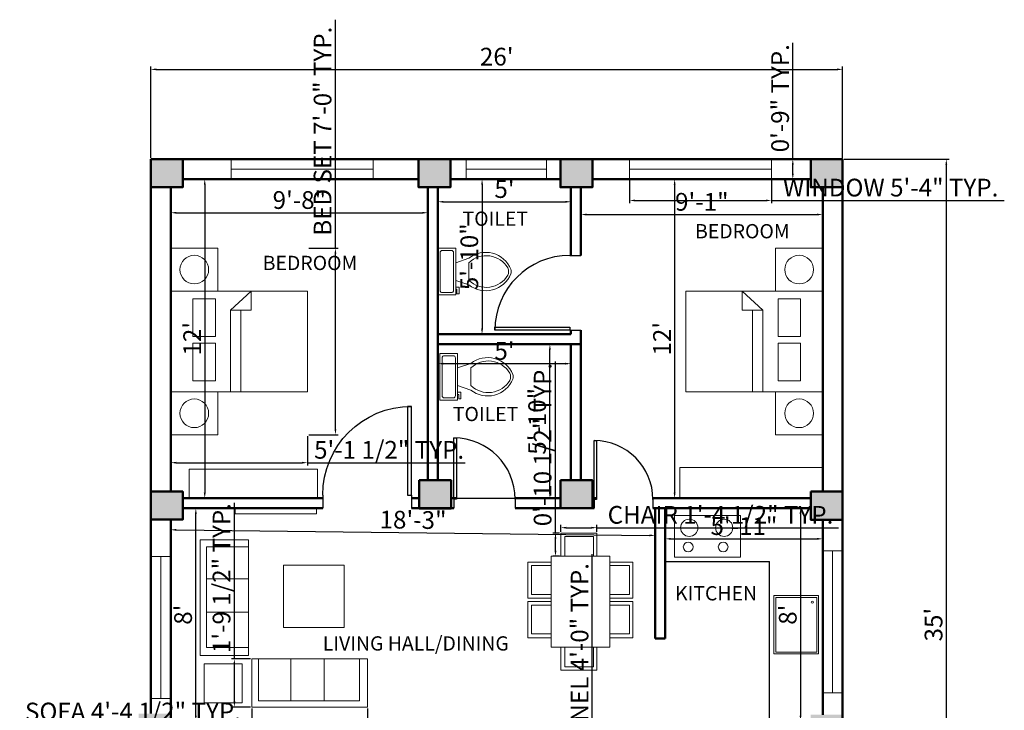
# Model space of a CAD drawing. Units: inches. Extents: x 716 to 1282, y 805 to 1949.
# Tile 2 of 2: x 716 to 1160, y 1009 to 1321. Entities that reach past the tile are written whole.
import ezdxf

# ---------------------------------------------------------------- set-up
doc = ezdxf.new("R2010")
doc.units = ezdxf.units.IN
for name, color, linetype, lineweight in [('A-ANNO-DIMS', 2, 'Continuous', 18), ('A-AREA-IDEN', 10, 'Continuous', 25), ('A-COLS', 7, 'Continuous', 50), ('A-COLS-PATT', 252, 'Continuous', 13), ('A-DOOR', 3, 'Continuous', 25), ('A-EQPM', 8, 'Continuous', 18), ('A-FLOR-CASE', 32, 'Continuous', 25), ('A-FLOR-FIXT', 9, 'Continuous', 18), ('A-FURN', 8, 'Continuous', 18), ('A-GLAZ', 4, 'Continuous', 18), ('WALL', 150, 'Continuous', 50)]:
    doc.layers.add(name, color=color, linetype=linetype, lineweight=lineweight)
doc.styles.get("Standard").update_dxf_attribs({"font": 'arial.ttf'})
doc.dimstyles.new('ISO-25', dxfattribs={"dimtxt": 8, "dimasz": 2.5, "dimexe": 1.25, "dimexo": 0.625, "dimtad": 1, "dimdec": 0, "dimlunit": 4, "dimtxsty": 'Standard', "dimcen": 2.5, "dimadec": 0, "dimazin": 0, "dimtfac": 1, "dimtdec": 0, "dimtmove": 0, "dimatfit": 3, "dimfxl": 1, "dimarcsym": 0})

# ---------------------------------------------------------------- blocks, each defined once
blk = doc.blocks.new('*U4')
for p, q in [((9.5, -6), (9.5, -2)), ((-10, -8.5), (-8, -8.5)), ((-10, -9.5), (-10, -8.5)), ((-8, -8.5), (-8, -8)), ((-7, -8), (-7, -9.5)), ((-4, -8), (-6, -14)), ((4, -8), (6, -14)), ((-7, -9.5), (-10, -9.5)), ((4, -14), (-4, -14))]:
    blk.add_line(p, q)
blk.add_lwpolyline([(10.5, -8), (10.5, 0), (-10.5, 0), (-10.5, -8)], close=True)
for points in [[(-9.5, -2), (-9.5, -6)], [(8.5, -1), (-8.5, -1)], [(-8.5, -7), (8.5, -7)]]:
    blk.add_lwpolyline(points)
for centre, radius, start, end in [((-8.62, -1.88), 0.884, 81.8699, 188.1301), ((8.62, -1.88), 0.884, 351.8699, 98.1301), ((-8.62, -6.12), 0.884, 171.8699, 278.1301), ((8.62, -6.12), 0.884, 261.8699, 8.1301), ((3.52, -21.58), 12.17, 141.4691, 247.9714), ((4.2, -21.82), 11.33, 136.3677, 238.9468), ((-3.52, -21.58), 12.17, 292.0284, 38.5307), ((-4.2, -21.82), 11.33, 301.053, 43.6321), ((0, -27.88), 4, 245.7318, 294.2682), ((0, -29), 4, 254.8605, 285.1395)]:
    blk.add_arc(centre, radius, start, end)
blk = doc.blocks.new('*U2')
for p, q in [((0, 0), (0, -6)), ((40, 0), (40, -6))]:
    blk.add_line(p, q)
blk.add_lwpolyline([(0, 0), (0, 40), (1.75, 40), (1.75, 0)], close=True)
blk.add_arc((0, 0), 40, 0, 90)
blk = doc.blocks.new('*D5')
at = {"layer": 'A-ANNO-DIMS', "color": 0, "lineweight": -2, "transparency": 16777216}
for p, q in [((775.39, 1258.32), (775.39, 1299.47)), ((777.89, 1298.22), (1084.89, 1298.22)), ((1087.39, 1258.32), (1087.39, 1299.47))]:
    blk.add_line(p, q, dxfattribs=at)
at = {"layer": 'A-ANNO-DIMS', "color": 0, "transparency": 16777216}
for points in [[(777.89, 1298.64), (777.89, 1297.81), (775.39, 1298.22)], [(1084.89, 1298.64), (1084.89, 1297.81), (1087.39, 1298.22)]]:
    blk.add_solid(points, dxfattribs=at)
at = {"layer": 'Defpoints', "color": 0, "transparency": 16777216}
for p in [(1087.39, 1298.22), (775.39, 1257.69), (1087.39, 1257.69)]:
    blk.add_point(p, dxfattribs=at)
at = {"layer": 'A-ANNO-DIMS', "color": 0, "transparency": 16777216, "insert": (931.39, 1302.93), "char_height": 8, "attachment_point": 5}
blk.add_mtext("26'", dxfattribs=at)
blk = doc.blocks.new('*D6')
at = {"layer": 'A-ANNO-DIMS', "color": 0, "lineweight": -2, "transparency": 16777216}
for p, q in [((1088.02, 1257.69), (1135.39, 1257.69)), ((1134.14, 1255.19), (1134.14, 840.19)), ((1088.02, 837.69), (1135.39, 837.69))]:
    blk.add_line(p, q, dxfattribs=at)
at = {"layer": 'A-ANNO-DIMS', "color": 0, "transparency": 16777216}
for points in [[(1133.72, 1255.19), (1134.55, 1255.19), (1134.14, 1257.69)], [(1133.72, 840.19), (1134.55, 840.19), (1134.14, 837.69)]]:
    blk.add_solid(points, dxfattribs=at)
at = {"layer": 'Defpoints', "color": 0, "transparency": 16777216}
for p in [(1087.39, 1257.69), (1087.39, 837.69), (1134.14, 837.69)]:
    blk.add_point(p, dxfattribs=at)
at = {"layer": 'A-ANNO-DIMS', "color": 0, "transparency": 16777216, "insert": (1129.42, 1047.69), "char_height": 8, "attachment_point": 5, "rotation": 90}
blk.add_mtext("35'", dxfattribs=at)
blk = doc.blocks.new('*D7')
at = {"layer": 'A-ANNO-DIMS', "color": 0, "lineweight": -2, "transparency": 16777216}
for p, q in [((784.39, 1244.38), (784.39, 1232.29)), ((900.39, 1244.38), (900.39, 1232.29)), ((786.89, 1233.54), (897.89, 1233.54))]:
    blk.add_line(p, q, dxfattribs=at)
at = {"layer": 'A-ANNO-DIMS', "color": 0, "transparency": 16777216}
for points in [[(786.89, 1233.95), (786.89, 1233.12), (784.39, 1233.54)], [(897.89, 1233.95), (897.89, 1233.12), (900.39, 1233.54)]]:
    blk.add_solid(points, dxfattribs=at)
at = {"layer": 'Defpoints', "color": 0, "transparency": 16777216}
for p in [(784.39, 1245.01), (900.39, 1245.01), (900.39, 1233.54)]:
    blk.add_point(p, dxfattribs=at)
at = {"layer": 'A-ANNO-DIMS', "color": 0, "transparency": 16777216, "insert": (842.39, 1238.25), "char_height": 8, "attachment_point": 5}
blk.add_mtext('9\'-8"', dxfattribs=at)
blk = doc.blocks.new('*D8')
at = {"layer": 'A-ANNO-DIMS', "color": 0, "lineweight": -2, "transparency": 16777216}
for p, q in [((790.42, 1248.69), (800.98, 1248.69)), ((799.73, 1246.19), (799.73, 1107.19)), ((790.42, 1104.69), (800.98, 1104.69))]:
    blk.add_line(p, q, dxfattribs=at)
at = {"layer": 'A-ANNO-DIMS', "color": 0, "transparency": 16777216}
for points in [[(799.31, 1246.19), (800.14, 1246.19), (799.73, 1248.69)], [(799.31, 1107.19), (800.14, 1107.19), (799.73, 1104.69)]]:
    blk.add_solid(points, dxfattribs=at)
at = {"layer": 'Defpoints', "color": 0, "transparency": 16777216}
for p in [(789.79, 1248.69), (789.79, 1104.69), (799.73, 1104.69)]:
    blk.add_point(p, dxfattribs=at)
at = {"layer": 'A-ANNO-DIMS', "color": 0, "transparency": 16777216, "insert": (795.09, 1176.69), "char_height": 8, "attachment_point": 5, "rotation": 90}
blk.add_mtext("12'", dxfattribs=at)
blk = doc.blocks.new('*D9')
at = {"layer": 'A-ANNO-DIMS', "color": 0, "lineweight": -2, "transparency": 16777216}
for p, q in [((904.89, 1244.38), (904.89, 1237.25)), ((964.89, 1244.38), (964.89, 1237.25)), ((907.39, 1238.5), (962.39, 1238.5))]:
    blk.add_line(p, q, dxfattribs=at)
at = {"layer": 'A-ANNO-DIMS', "color": 0, "transparency": 16777216}
for points in [[(907.39, 1238.91), (907.39, 1238.08), (904.89, 1238.5)], [(962.39, 1238.91), (962.39, 1238.08), (964.89, 1238.5)]]:
    blk.add_solid(points, dxfattribs=at)
at = {"layer": 'Defpoints', "color": 0, "transparency": 16777216}
for p in [(904.89, 1245.01), (964.89, 1245.01), (964.89, 1238.5)]:
    blk.add_point(p, dxfattribs=at)
at = {"layer": 'A-ANNO-DIMS', "color": 0, "transparency": 16777216, "insert": (934.89, 1243.19), "char_height": 8, "attachment_point": 5}
blk.add_mtext("5'", dxfattribs=at)
blk = doc.blocks.new('*D10')
at = {"layer": 'A-ANNO-DIMS', "color": 0, "lineweight": -2, "transparency": 16777216}
for p, q in [((911.42, 1174.19), (956.62, 1174.19)), ((955.37, 1107.19), (955.37, 1171.69)), ((911.42, 1104.69), (956.62, 1104.69))]:
    blk.add_line(p, q, dxfattribs=at)
at = {"layer": 'A-ANNO-DIMS', "color": 0, "transparency": 16777216}
for points in [[(954.95, 1171.69), (955.78, 1171.69), (955.37, 1174.19)], [(954.95, 1107.19), (955.78, 1107.19), (955.37, 1104.69)]]:
    blk.add_solid(points, dxfattribs=at)
at = {"layer": 'Defpoints', "color": 0, "transparency": 16777216}
for p in [(910.8, 1174.19), (955.37, 1174.19), (910.8, 1104.69)]:
    blk.add_point(p, dxfattribs=at)
at = {"layer": 'A-ANNO-DIMS', "color": 0, "transparency": 16777216, "insert": (950.66, 1139.44), "char_height": 8, "attachment_point": 5, "rotation": 90}
blk.add_mtext('5\'-10"', dxfattribs=at)
blk = doc.blocks.new('*D11')
at = {"layer": 'A-ANNO-DIMS', "color": 0, "lineweight": -2, "transparency": 16777216}
for p, q in [((911.16, 1248.69), (926.03, 1248.69)), ((924.78, 1246.19), (924.78, 1181.19)), ((911.16, 1178.69), (926.03, 1178.69))]:
    blk.add_line(p, q, dxfattribs=at)
at = {"layer": 'A-ANNO-DIMS', "color": 0, "transparency": 16777216}
for points in [[(924.37, 1246.19), (925.2, 1246.19), (924.78, 1248.69)], [(924.37, 1181.19), (925.2, 1181.19), (924.78, 1178.69)]]:
    blk.add_solid(points, dxfattribs=at)
at = {"layer": 'Defpoints', "color": 0, "transparency": 16777216}
for p in [(910.54, 1248.69), (910.54, 1178.69), (924.78, 1178.69)]:
    blk.add_point(p, dxfattribs=at)
at = {"layer": 'A-ANNO-DIMS', "color": 0, "transparency": 16777216, "insert": (920.07, 1213.69), "char_height": 8, "attachment_point": 5, "rotation": 90}
blk.add_mtext('5\'-10"', dxfattribs=at)
blk = doc.blocks.new('*D12')
at = {"layer": 'A-ANNO-DIMS', "color": 0, "lineweight": -2, "transparency": 16777216}
for p, q in [((904.89, 1173.57), (904.89, 1164.2)), ((964.89, 1171.57), (964.89, 1164.2)), ((907.39, 1165.45), (962.39, 1165.45))]:
    blk.add_line(p, q, dxfattribs=at)
at = {"layer": 'A-ANNO-DIMS', "color": 0, "transparency": 16777216}
for points in [[(907.39, 1165.87), (907.39, 1165.03), (904.89, 1165.45)], [(962.39, 1165.87), (962.39, 1165.03), (964.89, 1165.45)]]:
    blk.add_solid(points, dxfattribs=at)
at = {"layer": 'Defpoints', "color": 0, "transparency": 16777216}
for p in [(904.89, 1174.19), (964.89, 1172.2), (964.89, 1165.45)]:
    blk.add_point(p, dxfattribs=at)
at = {"layer": 'A-ANNO-DIMS', "color": 0, "transparency": 16777216, "insert": (934.89, 1170.14), "char_height": 8, "attachment_point": 5}
blk.add_mtext("5'", dxfattribs=at)
blk = doc.blocks.new('*D13')
at = {"layer": 'A-ANNO-DIMS', "color": 0, "lineweight": -2, "transparency": 16777216}
for p, q in [((969.39, 1244.38), (969.39, 1231.47)), ((1078.39, 1244.38), (1078.39, 1231.47)), ((971.89, 1232.72), (1075.89, 1232.72))]:
    blk.add_line(p, q, dxfattribs=at)
at = {"layer": 'A-ANNO-DIMS', "color": 0, "transparency": 16777216}
for points in [[(971.89, 1233.14), (971.89, 1232.31), (969.39, 1232.72)], [(1075.89, 1233.14), (1075.89, 1232.31), (1078.39, 1232.72)]]:
    blk.add_solid(points, dxfattribs=at)
at = {"layer": 'Defpoints', "color": 0, "transparency": 16777216}
for p in [(969.39, 1245.01), (1078.39, 1245.01), (1078.39, 1232.72)]:
    blk.add_point(p, dxfattribs=at)
at = {"layer": 'A-ANNO-DIMS', "color": 0, "transparency": 16777216, "insert": (1023.89, 1237.43), "char_height": 8, "attachment_point": 5}
blk.add_mtext('9\'-1"', dxfattribs=at)
blk = doc.blocks.new('*D14')
at = {"layer": 'A-ANNO-DIMS', "color": 0, "lineweight": -2, "transparency": 16777216}
for p, q in [((1072.37, 1248.69), (1010.37, 1248.69)), ((1011.62, 1246.19), (1011.62, 1107.19)), ((1072.37, 1104.69), (1010.37, 1104.69))]:
    blk.add_line(p, q, dxfattribs=at)
at = {"layer": 'A-ANNO-DIMS', "color": 0, "transparency": 16777216}
for points in [[(1011.21, 1246.19), (1012.04, 1246.19), (1011.62, 1248.69)], [(1011.21, 1107.19), (1012.04, 1107.19), (1011.62, 1104.69)]]:
    blk.add_solid(points, dxfattribs=at)
at = {"layer": 'Defpoints', "color": 0, "transparency": 16777216}
for p in [(1072.99, 1248.69), (1011.62, 1104.69), (1072.99, 1104.69)]:
    blk.add_point(p, dxfattribs=at)
at = {"layer": 'A-ANNO-DIMS', "color": 0, "transparency": 16777216, "insert": (1006.98, 1176.69), "char_height": 8, "attachment_point": 5, "rotation": 90}
blk.add_mtext("12'", dxfattribs=at)
blk = doc.blocks.new('*D15')
at = {"layer": 'A-ANNO-DIMS', "color": 0, "lineweight": -2, "transparency": 16777216}
for p, q in [((1007.39, 1042.03), (1007.39, 1087.66)), ((1009.89, 1086.41), (1075.89, 1086.41)), ((1078.39, 1042.03), (1078.39, 1087.66))]:
    blk.add_line(p, q, dxfattribs=at)
at = {"layer": 'A-ANNO-DIMS', "color": 0, "transparency": 16777216}
for points in [[(1009.89, 1086.82), (1009.89, 1085.99), (1007.39, 1086.41)], [(1075.89, 1086.82), (1075.89, 1085.99), (1078.39, 1086.41)]]:
    blk.add_solid(points, dxfattribs=at)
at = {"layer": 'Defpoints', "color": 0, "transparency": 16777216}
for p in [(1078.39, 1086.41), (1007.39, 1041.41), (1078.39, 1041.41)]:
    blk.add_point(p, dxfattribs=at)
at = {"layer": 'A-ANNO-DIMS', "color": 0, "transparency": 16777216, "insert": (1042.89, 1091.12), "char_height": 8, "attachment_point": 5}
blk.add_mtext('5\'-11"', dxfattribs=at)
blk = doc.blocks.new('*D16')
at = {"layer": 'A-ANNO-DIMS', "color": 0, "lineweight": -2, "transparency": 16777216}
for p, q in [((1072.37, 1100.19), (1067.14, 1100.19)), ((1068.39, 1097.69), (1068.39, 1006.69)), ((1072.37, 1004.19), (1067.14, 1004.19))]:
    blk.add_line(p, q, dxfattribs=at)
at = {"layer": 'A-ANNO-DIMS', "color": 0, "transparency": 16777216}
for points in [[(1067.97, 1097.69), (1068.8, 1097.69), (1068.39, 1100.19)], [(1067.97, 1006.69), (1068.8, 1006.69), (1068.39, 1004.19)]]:
    blk.add_solid(points, dxfattribs=at)
at = {"layer": 'Defpoints', "color": 0, "transparency": 16777216}
for p in [(1072.99, 1100.19), (1068.39, 1004.19), (1072.99, 1004.19)]:
    blk.add_point(p, dxfattribs=at)
at = {"layer": 'A-ANNO-DIMS', "color": 0, "transparency": 16777216, "insert": (1063.68, 1052.19), "char_height": 8, "attachment_point": 5, "rotation": 90}
blk.add_mtext("8'", dxfattribs=at)
blk = doc.blocks.new('*D24')
at = {"layer": 'A-ANNO-DIMS', "color": 0, "lineweight": -2, "transparency": 16777216}
for p, q in [((848.65, 1100.19), (794.45, 1100.19)), ((795.7, 1006.69), (795.7, 1097.69)), ((848.65, 1004.19), (794.45, 1004.19))]:
    blk.add_line(p, q, dxfattribs=at)
at = {"layer": 'A-ANNO-DIMS', "color": 0, "transparency": 16777216}
for points in [[(795.28, 1097.69), (796.11, 1097.69), (795.7, 1100.19)], [(795.28, 1006.69), (796.11, 1006.69), (795.7, 1004.19)]]:
    blk.add_solid(points, dxfattribs=at)
at = {"layer": 'Defpoints', "color": 0, "transparency": 16777216}
for p in [(795.7, 1100.19), (849.27, 1100.19), (849.27, 1004.19)]:
    blk.add_point(p, dxfattribs=at)
at = {"layer": 'A-ANNO-DIMS', "color": 0, "transparency": 16777216, "insert": (790.99, 1052.19), "char_height": 8, "attachment_point": 5, "rotation": 90}
blk.add_mtext("8'", dxfattribs=at)
blk = doc.blocks.new('*D25')
at = {"layer": 'A-ANNO-DIMS', "color": 0, "lineweight": -2, "transparency": 16777216}
for p, q in [((784.39, 1094.45), (784.32, 1089.25)), ((786.84, 1090.47), (1000.34, 1087.98)), ((1002.89, 1091.9), (1002.82, 1086.7))]:
    blk.add_line(p, q, dxfattribs=at)
at = {"layer": 'A-ANNO-DIMS', "color": 0, "transparency": 16777216}
for points in [[(786.84, 1090.89), (786.83, 1090.05), (784.34, 1090.5)], [(1000.34, 1088.4), (1000.33, 1087.56), (1002.84, 1087.95)]]:
    blk.add_solid(points, dxfattribs=at)
at = {"layer": 'Defpoints', "color": 0, "transparency": 16777216}
for p in [(784.39, 1095.07), (1002.89, 1092.52), (1002.84, 1087.95)]:
    blk.add_point(p, dxfattribs=at)
at = {"layer": 'A-ANNO-DIMS', "color": 0, "transparency": 16777216, "insert": (893.64, 1093.94), "char_height": 8, "attachment_point": 5, "rotation": 359.331}
blk.add_mtext('18\'-3"', dxfattribs=at)
blk = doc.blocks.new('BED-DOUBLE-WITH-NIGHTSTANDS')
for p, q in [((36.29, 64.82), (27, 56.14)), ((36.29, 56.14), (36.29, 64.82)), ((27, 19.35), (27, 56.14)), ((27, 56.14), (36.29, 56.14)), ((31.64, 56.14), (31.64, 19.35))]:
    blk.add_line(p, q)
for points in [[(0, 64.82), (21.22, 64.82), (21.22, 84.17), (0, 84.17)], [(0, 64.82), (61.64, 64.82), (61.64, 19.35), (0, 19.35)], [(9.94, 44.27), (20.15, 44.27), (20.15, 61.31), (9.94, 61.31)], [(9.94, 24.34), (20.15, 24.34), (20.15, 41.38), (9.94, 41.38)], [(0, 0), (21.22, 0), (21.22, 19.35), (0, 19.35)]]:
    blk.add_lwpolyline(points, close=True)
for centre in [(10.61, 74.5), (10.61, 9.67)]:
    blk.add_circle(centre, 6.48)
blk = doc.blocks.new('SOFA-THREE-SEAT')
for p, q in [((21.72, 52.25), (0, 52.25)), ((0, 52.25), (0, 0)), ((21.72, 49.16), (21.72, 52.25)), ((2.8, 34.63), (21.72, 34.63)), ((2.8, 19.65), (21.72, 19.65)), ((0, 0), (21.72, 0)), ((21.72, 0), (21.72, 3.64))]:
    blk.add_line(p, q)
blk.add_lwpolyline([(2.8, 49.16), (21.72, 49.16), (21.72, 3.64), (2.8, 3.64)], close=True)
blk = doc.blocks.new('CHAIR-DINING')
for p, q in [((0, 0), (0, 10.47)), ((0, 10.47), (16.26, 10.47)), ((16.26, 10.47), (16.26, 0))]:
    blk.add_line(p, q)
blk.add_lwpolyline([(1.72, 0), (14.73, 0), (14.73, 8.87), (1.72, 8.87)], close=True)
blk = doc.blocks.new('WINDOW-64IN')
blk.add_line((0, 4.5), (64.04, 4.5))
blk.add_lwpolyline([(0, 9), (64.04, 9), (64.04, 0), (0, 0)], close=True)
blk = doc.blocks.new('*D31')
at = {"layer": 'A-ANNO-DIMS', "color": 0, "lineweight": -2, "transparency": 16777216}
for p, q in [((858.66, 1217.56), (858.66, 1320.65)), ((846.66, 1217.56), (859.91, 1217.56)), ((858.66, 1135.89), (858.66, 1215.06)), ((846.66, 1133.39), (859.91, 1133.39))]:
    blk.add_line(p, q, dxfattribs=at)
at = {"layer": 'A-ANNO-DIMS', "color": 0, "transparency": 16777216}
for points in [[(858.24, 1215.06), (859.08, 1215.06), (858.66, 1217.56)], [(858.24, 1135.89), (859.08, 1135.89), (858.66, 1133.39)]]:
    blk.add_solid(points, dxfattribs=at)
at = {"layer": 'Defpoints', "color": 0, "transparency": 16777216}
for p in [(846.04, 1217.56), (858.66, 1217.56), (846.04, 1133.39)]:
    blk.add_point(p, dxfattribs=at)
at = {"layer": 'A-ANNO-DIMS', "color": 0, "transparency": 16777216, "insert": (853.9, 1270.35), "char_height": 8, "attachment_point": 5, "rotation": 90}
blk.add_mtext('BED SET 7\'-0" TYP.', dxfattribs=at)
blk = doc.blocks.new('*D32')
at = {"layer": 'A-ANNO-DIMS', "color": 0, "lineweight": -2, "transparency": 16777216}
for p, q in [((784.39, 1132.77), (784.39, 1119.52)), ((846.04, 1132.77), (846.04, 1119.52)), ((786.89, 1120.77), (843.54, 1120.77)), ((846.04, 1120.77), (917.19, 1120.77))]:
    blk.add_line(p, q, dxfattribs=at)
at = {"layer": 'A-ANNO-DIMS', "color": 0, "transparency": 16777216}
for points in [[(786.89, 1121.18), (786.89, 1120.35), (784.39, 1120.77)], [(843.54, 1121.18), (843.54, 1120.35), (846.04, 1120.77)]]:
    blk.add_solid(points, dxfattribs=at)
at = {"layer": 'Defpoints', "color": 0, "transparency": 16777216}
for p in [(784.39, 1133.39), (846.04, 1133.39), (846.04, 1120.77)]:
    blk.add_point(p, dxfattribs=at)
at = {"layer": 'A-ANNO-DIMS', "color": 0, "transparency": 16777216, "insert": (882.86, 1125.53), "char_height": 8, "attachment_point": 5}
blk.add_mtext('5\'-1 1/2" TYP.', dxfattribs=at)
blk = doc.blocks.new('*D33')
at = {"layer": 'A-ANNO-DIMS', "color": 0, "lineweight": -2, "transparency": 16777216}
for p, q in [((820.93, 1009.9), (820.93, 1001.44)), ((873.18, 1009.9), (873.18, 1001.44)), ((820.93, 1002.69), (716.28, 1002.69)), ((870.68, 1002.69), (823.43, 1002.69))]:
    blk.add_line(p, q, dxfattribs=at)
at = {"layer": 'A-ANNO-DIMS', "color": 0, "transparency": 16777216}
for points in [[(823.43, 1003.11), (823.43, 1002.27), (820.93, 1002.69)], [(870.68, 1003.11), (870.68, 1002.27), (873.18, 1002.69)]]:
    blk.add_solid(points, dxfattribs=at)
at = {"layer": 'Defpoints', "color": 0, "transparency": 16777216}
for p in [(820.93, 1010.53), (873.18, 1010.53), (820.93, 1002.69)]:
    blk.add_point(p, dxfattribs=at)
at = {"layer": 'A-ANNO-DIMS', "color": 0, "transparency": 16777216, "insert": (767.35, 1007.45), "char_height": 8, "attachment_point": 5}
blk.add_mtext('SOFA 4\'-4 1/2" TYP.', dxfattribs=at)
blk = doc.blocks.new('*D34')
at = {"layer": 'A-ANNO-DIMS', "color": 0, "lineweight": -2, "transparency": 16777216}
for p, q in [((813.09, 1032.24), (813.09, 1102.65)), ((820.3, 1032.24), (811.84, 1032.24)), ((813.09, 1013.03), (813.09, 1029.74)), ((820.3, 1010.53), (811.84, 1010.53))]:
    blk.add_line(p, q, dxfattribs=at)
at = {"layer": 'A-ANNO-DIMS', "color": 0, "transparency": 16777216}
for points in [[(812.67, 1029.74), (813.5, 1029.74), (813.09, 1032.24)], [(812.67, 1013.03), (813.5, 1013.03), (813.09, 1010.53)]]:
    blk.add_solid(points, dxfattribs=at)
at = {"layer": 'Defpoints', "color": 0, "transparency": 16777216}
for p in [(813.09, 1032.24), (820.93, 1032.24), (820.93, 1010.53)]:
    blk.add_point(p, dxfattribs=at)
at = {"layer": 'A-ANNO-DIMS', "color": 0, "transparency": 16777216, "insert": (808.33, 1068.7), "char_height": 8, "attachment_point": 5, "rotation": 90}
blk.add_mtext('1\'-9 1/2" TYP.', dxfattribs=at)
blk = doc.blocks.new('*D35')
at = {"layer": 'A-ANNO-DIMS', "color": 0, "lineweight": -2, "transparency": 16777216}
for p, q in [((974.5, 953.37), (974.5, 1079.51)), ((967.94, 953.37), (975.75, 953.37)), ((974.5, 907.97), (974.5, 950.87)), ((967.94, 905.47), (975.75, 905.47))]:
    blk.add_line(p, q, dxfattribs=at)
at = {"layer": 'A-ANNO-DIMS', "color": 0, "transparency": 16777216}
for points in [[(974.08, 950.87), (974.92, 950.87), (974.5, 953.37)], [(974.08, 907.97), (974.92, 907.97), (974.5, 905.47)]]:
    blk.add_solid(points, dxfattribs=at)
at = {"layer": 'Defpoints', "color": 0, "transparency": 16777216}
for p in [(967.31, 953.37), (974.5, 953.37), (967.31, 905.47)]:
    blk.add_point(p, dxfattribs=at)
at = {"layer": 'A-ANNO-DIMS', "color": 0, "transparency": 16777216, "insert": (969.79, 1017.69), "char_height": 8, "attachment_point": 5, "rotation": 90}
blk.add_mtext('WALL PANEL 4\'-0" TYP.', dxfattribs=at)
blk = doc.blocks.new('*D37')
at = {"layer": 'A-ANNO-DIMS', "color": 0, "lineweight": -2, "transparency": 16777216}
for p, q in [((991.27, 1248.07), (991.27, 1237.84)), ((1055.31, 1248.07), (1055.31, 1237.84)), ((993.77, 1239.09), (1052.81, 1239.09)), ((1055.31, 1239.09), (1160.29, 1239.09))]:
    blk.add_line(p, q, dxfattribs=at)
at = {"layer": 'A-ANNO-DIMS', "color": 0, "transparency": 16777216}
for points in [[(993.77, 1239.5), (993.77, 1238.67), (991.27, 1239.09)], [(1052.81, 1239.5), (1052.81, 1238.67), (1055.31, 1239.09)]]:
    blk.add_solid(points, dxfattribs=at)
at = {"layer": 'Defpoints', "color": 0, "transparency": 16777216}
for p in [(991.27, 1248.69), (1055.31, 1248.69), (1055.31, 1239.09)]:
    blk.add_point(p, dxfattribs=at)
at = {"layer": 'A-ANNO-DIMS', "color": 0, "transparency": 16777216, "insert": (1109.05, 1243.85), "char_height": 8, "attachment_point": 5}
blk.add_mtext('WINDOW 5\'-4" TYP.', dxfattribs=at)
blk = doc.blocks.new('*D38')
at = {"layer": 'A-ANNO-DIMS', "color": 0, "lineweight": -2, "transparency": 16777216}
for p, q in [((1064.92, 1257.69), (1064.92, 1310.21)), ((1055.94, 1257.69), (1066.17, 1257.69)), ((1064.92, 1251.19), (1064.92, 1255.19)), ((1055.94, 1248.69), (1066.17, 1248.69))]:
    blk.add_line(p, q, dxfattribs=at)
at = {"layer": 'A-ANNO-DIMS', "color": 0, "transparency": 16777216}
for points in [[(1064.5, 1255.19), (1065.33, 1255.19), (1064.92, 1257.69)], [(1064.5, 1251.19), (1065.33, 1251.19), (1064.92, 1248.69)]]:
    blk.add_solid(points, dxfattribs=at)
at = {"layer": 'Defpoints', "color": 0, "transparency": 16777216}
for p in [(1055.31, 1257.69), (1064.92, 1257.69), (1055.31, 1248.69)]:
    blk.add_point(p, dxfattribs=at)
at = {"layer": 'A-ANNO-DIMS', "color": 0, "transparency": 16777216, "insert": (1060.21, 1285.2), "char_height": 8, "attachment_point": 5, "rotation": 90}
blk.add_mtext('0\'-9" TYP.', dxfattribs=at)
blk = doc.blocks.new('*D39')
at = {"layer": 'A-ANNO-DIMS', "color": 0, "lineweight": -2, "transparency": 16777216}
for p, q in [((960.33, 1089.62), (960.33, 1092.69)), ((976.59, 1089.62), (976.59, 1092.69)), ((962.83, 1091.44), (974.09, 1091.44)), ((976.59, 1091.44), (1085.53, 1091.44))]:
    blk.add_line(p, q, dxfattribs=at)
at = {"layer": 'A-ANNO-DIMS', "color": 0, "transparency": 16777216}
for points in [[(962.83, 1091.85), (962.83, 1091.02), (960.33, 1091.44)], [(974.09, 1091.85), (974.09, 1091.02), (976.59, 1091.44)]]:
    blk.add_solid(points, dxfattribs=at)
at = {"layer": 'Defpoints', "color": 0, "transparency": 16777216}
for p in [(960.33, 1089), (976.59, 1091.44), (976.59, 1089)]:
    blk.add_point(p, dxfattribs=at)
at = {"layer": 'A-ANNO-DIMS', "color": 0, "transparency": 16777216, "insert": (1032.31, 1096.2), "char_height": 8, "attachment_point": 5}
blk.add_mtext('CHAIR 1\'-4 1/2" TYP.', dxfattribs=at)
blk = doc.blocks.new('*D40')
at = {"layer": 'A-ANNO-DIMS', "color": 0, "lineweight": -2, "transparency": 16777216}
for p, q in [((957.9, 1089), (957.9, 1166.37)), ((959.71, 1089), (956.65, 1089)), ((957.9, 1081.03), (957.9, 1086.5)), ((959.71, 1078.53), (956.65, 1078.53))]:
    blk.add_line(p, q, dxfattribs=at)
at = {"layer": 'A-ANNO-DIMS', "color": 0, "transparency": 16777216}
for points in [[(957.48, 1086.5), (958.31, 1086.5), (957.9, 1089)], [(957.48, 1081.03), (958.31, 1081.03), (957.9, 1078.53)]]:
    blk.add_solid(points, dxfattribs=at)
at = {"layer": 'Defpoints', "color": 0, "transparency": 16777216}
for p in [(957.9, 1089), (960.33, 1089), (960.33, 1078.53)]:
    blk.add_point(p, dxfattribs=at)
at = {"layer": 'A-ANNO-DIMS', "color": 0, "transparency": 16777216, "insert": (953.13, 1128.93), "char_height": 8, "attachment_point": 5, "rotation": 90}
blk.add_mtext('0\'-10 1/2" TYP.', dxfattribs=at)

msp = doc.modelspace()

# ---------------------------------------------------------------- hatches: boundary and pattern name
at = {"layer": 'A-COLS-PATT'}
h = msp.add_hatch(color=256, dxfattribs=at)
h.dxf.hatch_style = 1
h.paths.add_polyline_path([(789.79, 1257.69), (775.39, 1257.69), (775.39, 1245.01), (789.79, 1245.01)])
h.paths.add_polyline_path([(910.54, 1257.69), (896.14, 1257.69), (896.14, 1245.01), (910.54, 1245.01)])
h.paths.add_polyline_path([(974.53, 1257.69), (960.13, 1257.69), (960.13, 1245.01), (974.53, 1245.01)])
h.paths.add_polyline_path([(1087.39, 1257.69), (1072.99, 1257.69), (1072.99, 1245.01), (1087.39, 1245.01)])
h.paths.add_polyline_path([(789.79, 1107.76), (775.39, 1107.76), (775.39, 1095.07), (789.79, 1095.07)])
h.paths.add_polyline_path([(784.39, 1007.56), (769.99, 1007.56), (769.99, 994.87), (784.39, 994.87)])
h.paths.add_polyline_path([(789.79, 883.38), (775.39, 883.38), (775.39, 870.69), (789.79, 870.69)])
h.paths.add_polyline_path([(789.79, 850.38), (775.39, 850.38), (775.39, 837.69), (789.79, 837.69)])
h.paths.add_polyline_path([(910.16, 850.38), (895.76, 850.38), (895.76, 837.69), (910.16, 837.69)])
h.paths.add_polyline_path([(908.09, 883.38), (893.69, 883.38), (893.69, 870.69), (908.09, 870.69)])
h.paths.add_polyline_path([(969.44, 883.38), (955.04, 883.38), (955.04, 870.69), (969.44, 870.69)])
h.paths.add_polyline_path([(969.95, 850.38), (955.55, 850.38), (955.55, 837.69), (969.95, 837.69)])
h.paths.add_polyline_path([(1087.39, 881.16), (1072.99, 881.16), (1072.99, 868.48), (1087.39, 868.48)])
h.paths.add_polyline_path([(1087.39, 850.38), (1072.99, 850.38), (1072.99, 837.69), (1087.39, 837.69)])
h.paths.add_polyline_path([(1087.39, 1007.07), (1072.99, 1007.07), (1072.99, 994.38), (1087.39, 994.38)])
h.paths.add_polyline_path([(972.29, 1004.19), (957.89, 1004.19), (957.89, 991.51), (972.29, 991.51)])
h.paths.add_polyline_path([(904.89, 1004.19), (890.49, 1004.19), (890.49, 991.51), (904.89, 991.51)])
h.paths.add_polyline_path([(974.58, 1112.88), (960.18, 1112.88), (960.18, 1100.19), (974.58, 1100.19)])
h.paths.add_polyline_path([(1087.39, 1107.7), (1072.99, 1107.7), (1072.99, 1095.02), (1087.39, 1095.02)])
h.paths.add_polyline_path([(910.8, 1112.82), (896.4, 1112.82), (896.4, 1100.19), (904.89, 1100.19), (910.8, 1100.19)])

# ---------------------------------------------------------------- linework, layer by layer
at = {"layer": 'A-COLS'}
for points in [[(775.39, 1257.69), (789.79, 1257.69), (789.79, 1245.01), (775.39, 1245.01)], [(896.14, 1257.69), (910.54, 1257.69), (910.54, 1245.01), (896.14, 1245.01)], [(960.13, 1257.69), (974.53, 1257.69), (974.53, 1245.01), (960.13, 1245.01)], [(1072.99, 1257.69), (1087.39, 1257.69), (1087.39, 1245.01), (1072.99, 1245.01)], [(896.4, 1112.82), (910.8, 1112.82), (910.8, 1100.13), (896.4, 1100.13)], [(960.18, 1112.88), (974.58, 1112.88), (974.58, 1100.19), (960.18, 1100.19)], [(775.39, 1107.76), (789.79, 1107.76), (789.79, 1095.07), (775.39, 1095.07)], [(1072.99, 1107.7), (1087.39, 1107.7), (1087.39, 1095.02), (1072.99, 1095.02)]]:
    msp.add_lwpolyline(points, close=True, dxfattribs=at)
at = {"layer": 'A-EQPM'}
msp.add_lwpolyline([(1011.5, 1096.92), (1041.32, 1096.92), (1041.32, 1078.13), (1011.5, 1078.13)], close=True, dxfattribs=at)
for centre, radius in [((1018.22, 1091.41), 3.88), ((1033.98, 1091.41), 3.88), ((1017.74, 1082.77), 2.2), ((1033.51, 1082.77), 2.2)]:
    msp.add_circle(centre, radius, dxfattribs=at)
at = {"layer": 'A-FLOR-CASE'}
for p, q in [((1007.39, 1100.19), (1007.39, 1076.19)), ((1007.39, 1076.19), (1054.39, 1076.19)), ((1054.39, 1004.19), (1054.39, 1076.19))]:
    msp.add_line(p, q, dxfattribs=at)
at = {"layer": 'A-FLOR-FIXT'}
for points in [[(1056.33, 1060.84), (1076.51, 1060.84), (1076.51, 1034.58), (1056.33, 1034.58)], [(1057.26, 1060), (1075.78, 1060), (1075.78, 1035.34), (1057.26, 1035.34)]]:
    msp.add_lwpolyline(points, close=True, dxfattribs=at)
msp.add_circle((1073.72, 1057.86), 0.473, dxfattribs=at)
at = {"layer": 'A-FURN'}
for points in [[(792.64, 1104.69), (850.56, 1104.69), (850.56, 1117.8), (792.64, 1117.8)], [(813.42, 1100.19), (850.12, 1100.19), (850.12, 1097.7), (813.42, 1097.7)], [(835.19, 1046.38), (862.67, 1046.38), (862.67, 1074.58), (835.19, 1074.58)], [(955.89, 1078.53), (982.35, 1078.53), (982.35, 1037.6), (955.89, 1037.6)], [(799.42, 1030.08), (816.65, 1030.08), (816.65, 1012.4), (799.42, 1012.4)]]:
    msp.add_lwpolyline(points, close=True, dxfattribs=at)
msp.add_lwpolyline([(1078.39, 1107.7), (1078.39, 1118.65), (1014.04, 1118.65), (1014.04, 1104.69), (1072.99, 1104.69)], dxfattribs=at)
at = {"layer": 'A-GLAZ'}
for p, q in [((917.65, 1253.19), (953.78, 1253.19)), ((1082.89, 1081.04), (1082.89, 1017))]:
    msp.add_line(p, q, dxfattribs=at)
for points in [[(917.65, 1257.69), (953.78, 1257.69), (953.78, 1248.69), (917.65, 1248.69)], [(1087.39, 1081.04), (1087.39, 1017), (1078.39, 1017), (1078.39, 1081.04)]]:
    msp.add_lwpolyline(points, close=True, dxfattribs=at)
at = {"layer": 'WALL'}
for p, q in [((775.39, 1257.69), (1087.39, 1257.69)), ((775.39, 1007.56), (775.39, 1257.69)), ((1087.39, 1257.69), (1087.39, 837.69)), ((789.79, 1248.69), (896.14, 1248.69)), ((789.79, 1248.69), (896.14, 1248.69)), ((910.54, 1248.69), (960.13, 1248.69)), ((910.54, 1248.69), (960.13, 1248.69)), ((974.53, 1248.69), (1072.99, 1248.69)), ((784.39, 1107.76), (784.39, 1245.01)), ((900.39, 1245.01), (900.39, 1112.82)), ((904.89, 1245.01), (904.89, 1112.82)), ((964.89, 1245.01), (964.89, 1214.29)), ((969.39, 1245.01), (969.39, 1214.29)), ((1078.39, 1245.01), (1078.39, 1107.7)), ((964.89, 1178.69), (904.89, 1178.69)), ((964.89, 1180.51), (964.89, 1178.69)), ((969.39, 1180.51), (969.39, 1174.19)), ((969.39, 1174.19), (904.89, 1174.19)), ((904.89, 1174.19), (964.89, 1174.19)), ((964.89, 1174.19), (964.89, 1112.88)), ((969.39, 1174.19), (969.39, 1112.88)), ((852.93, 1104.69), (789.79, 1104.69)), ((896.4, 1104.69), (892.93, 1104.69)), ((910.8, 1104.69), (913.29, 1104.69)), ((939.66, 1104.69), (960.18, 1104.69)), ((974.58, 1104.69), (976.44, 1104.69)), ((1001.84, 1104.69), (1072.99, 1104.69)), ((852.93, 1100.19), (789.79, 1100.19)), ((904.89, 1100.19), (892.93, 1100.19)), ((904.89, 1100.19), (912.08, 1100.19)), ((939.67, 1100.19), (969.39, 1100.19)), ((969.39, 1100.19), (975.28, 1100.19)), ((1001.84, 1100.19), (1072.99, 1100.19)), ((1002.89, 1100.19), (1002.89, 1041.41)), ((1072.99, 1100.19), (1007.39, 1100.19)), ((1007.39, 1100.19), (1007.39, 1041.41)), ((784.39, 1095.07), (784.39, 1004.19)), ((784.39, 883.38), (784.39, 1095.07)), ((1078.39, 1095.02), (1078.39, 1007.07)), ((1002.89, 1041.41), (1007.39, 1041.41))]:
    msp.add_line(p, q, dxfattribs=at)

# ---------------------------------------------------------------- block references
at = {"layer": 'A-DOOR', "xscale": 0.8444741693690019, "yscale": 0.8444741693690019, "zscale": 0.8444741693690019, "rotation": 90}
msp.add_blockref('*U2', (964.33, 1180.51), dxfattribs=at)
at = {"layer": 'A-DOOR', "xscale": -1}
msp.add_blockref('*U2', (892.93, 1106.19), dxfattribs=at)
at = {"layer": 'A-DOOR'}
for p, xscale, yscale, zscale in [((912.08, 1104.33), 0.689653487353441, 0.689653487353441, 0.689653487353441), ((975.28, 1104.18), 0.6640096988613329, 0.6640096988613329, 0.6640096988613329)]:
    msp.add_blockref('*U2', p, dxfattribs=dict(at, xscale=xscale, yscale=yscale, zscale=zscale))
at = {"layer": 'A-FLOR-FIXT', "rotation": 90}
for p in [(904.89, 1207), (905.77, 1159.54)]:
    msp.add_blockref('*U4', p, dxfattribs=at)
at = {"layer": 'A-FURN'}
for name, p in [('BED-DOUBLE-WITH-NIGHTSTANDS', (784.39, 1133.39)), ('CHAIR-DINING', (960.33, 1078.53)), ('SOFA-THREE-SEAT', (797.69, 1033.71))]:
    msp.add_blockref(name, p, dxfattribs=at)
at = {"layer": 'A-FURN', "extrusion": (0, 0, -1), "zscale": -1}
msp.add_blockref('BED-DOUBLE-WITH-NIGHTSTANDS', (-1078.39, 1133.39), dxfattribs=at)
at = {"layer": 'A-FURN'}
for name, p, rotation in [('CHAIR-DINING', (955.89, 1059.6), 90.0000000000019), ('CHAIR-DINING', (955.89, 1041.81), 90.0000000000019), ('SOFA-THREE-SEAT', (873.18, 1010.53), 89.99999999999883)]:
    msp.add_blockref(name, p, dxfattribs=dict(at, rotation=rotation))
at = {"layer": 'A-FURN', "extrusion": (0, 0, -1), "zscale": -1}
for p, rotation in [((-982.35, 1059.6), 90.00000000000296), ((-982.35, 1041.81), 90.00000000000296), ((-960.33, 1037.6), 180)]:
    msp.add_blockref('CHAIR-DINING', p, dxfattribs=dict(at, rotation=rotation))
at = {"layer": 'A-GLAZ'}
for p in [(811.64, 1248.69), (991.27, 1248.69)]:
    msp.add_blockref('WINDOW-64IN', p, dxfattribs=at)
at = {"layer": 'A-GLAZ', "rotation": 270}
msp.add_blockref('WINDOW-64IN', (775.39, 1078.43), dxfattribs=at)

# ---------------------------------------------------------------- texts
at = {"layer": 'A-AREA-IDEN', "attachment_point": 1}
for s, insert, char_height in [('TOILET', (915.99, 1234.08), 6.429), ('BEDROOM', (1020.83, 1228.43), 6.429), ('BEDROOM', (825.87, 1214.11), 6.429), ('TOILET', (911.6, 1145.96), 6.429), ('KITCHEN', (1011.82, 1065.06), 6.429), ('LIVING HALL/DINING', (852.97, 1042.44), 6.4286)]:
    msp.add_mtext_dynamic_manual_height_columns(s, width=131.2996, gutter_width=32.14, heights=[0], dxfattribs=dict(at, insert=insert, char_height=char_height))

# ---------------------------------------------------------------- dimensions: what is measured, and where the dimension line sits
at = {"layer": 'A-ANNO-DIMS'}
for base, p1, p2, angle, text, picture, middle in [((858.66, 1217.56), (846.04, 1133.39), (846.04, 1217.56), 90, 'BED SET <> TYP.', '*D31', (853.9, 1270.35)), ((1064.92, 1257.69), (1055.31, 1248.69), (1055.31, 1257.69), 90, '<> TYP.', '*D38', (1060.21, 1285.2)), ((957.9, 1089), (960.33, 1078.53), (960.33, 1089), 90, '<> TYP.', '*D40', (953.13, 1128.93)), ((813.09, 1032.24), (820.93, 1010.53), (820.93, 1032.24), 90, '<> TYP.', '*D34', (808.33, 1068.7)), ((974.5, 953.37), (967.31, 905.47), (967.31, 953.37), 90, 'WALL PANEL <> TYP.', '*D35', (969.79, 1017.69)), ((820.9255, 1002.6901), (873.1788, 1010.5281), (820.9255, 1010.5281), 180, 'SOFA <> TYP.', '*D33', (767.3503, 1007.4543))]:
    dim = msp.add_linear_dim(base=base, p1=p1, p2=p2, angle=angle, text=text, dimstyle='ISO-25', override={"dimdec": 1, "dimlfac": 1, "dimrnd": 0, "dimzin": 1, "dimdsep": 46, "dimlunit": 4, "dimfrac": 2}, dxfattribs=at)
    dim.commit()
    dim.dimension.update_dxf_attribs({"geometry": picture, "text_midpoint": middle})
for base, p1, p2, picture, middle in [((1087.39, 1298.22), (775.39, 1257.69), (1087.39, 1257.69), '*D5', (931.39, 1302.93)), ((964.89, 1238.5), (904.89, 1245.01), (964.89, 1245.01), '*D9', (934.89, 1243.19)), ((900.39, 1233.54), (784.39, 1245.01), (900.39, 1245.01), '*D7', (842.39, 1238.25)), ((1078.39, 1232.72), (969.39, 1245.01), (1078.39, 1245.01), '*D13', (1023.89, 1237.43)), ((964.89, 1165.45), (904.89, 1174.19), (964.89, 1172.2), '*D12', (934.89, 1170.14)), ((1078.39, 1086.41), (1007.39, 1041.41), (1078.39, 1041.41), '*D15', (1042.89, 1091.12))]:
    dim = msp.add_linear_dim(base=base, p1=p1, p2=p2, dimstyle='ISO-25', override={"dimclrd": 0, "dimclre": 0, "dimclrt": 0}, dxfattribs=at)
    dim.commit()
    dim.dimension.update_dxf_attribs({"geometry": picture, "text_midpoint": middle})
for base, p1, p2, text, picture, middle in [((1055.31, 1239.09), (991.27, 1248.69), (1055.31, 1248.69), 'WINDOW <> TYP.', '*D37', (1109.05, 1243.85)), ((846.0356, 1120.767), (784.3926, 1133.3926), (846.0356, 1133.3926), '<> TYP.', '*D32', (882.8632, 1125.5284)), ((976.59, 1091.44), (960.33, 1089), (976.59, 1089), 'CHAIR <> TYP.', '*D39', (1032.31, 1096.2))]:
    dim = msp.add_linear_dim(base=base, p1=p1, p2=p2, text=text, dimstyle='ISO-25', override={"dimdec": 1, "dimlfac": 1, "dimrnd": 0, "dimzin": 1, "dimdsep": 46, "dimlunit": 4, "dimfrac": 2}, dxfattribs=at)
    dim.commit()
    dim.dimension.update_dxf_attribs({"geometry": picture, "text_midpoint": middle})
for base, p1, p2, picture, middle in [((1134.14, 837.69), (1087.39, 1257.69), (1087.39, 837.69), '*D6', (1129.42, 1047.69)), ((799.73, 1104.69), (789.79, 1248.69), (789.79, 1104.69), '*D8', (795.09, 1176.69)), ((924.78, 1178.69), (910.54, 1248.69), (910.54, 1178.69), '*D11', (920.07, 1213.69)), ((1011.62, 1104.69), (1072.99, 1248.69), (1072.99, 1104.69), '*D14', (1006.98, 1176.69)), ((955.36692195, 1174.19156326), (910.79514707, 1104.69156326), (910.79514707, 1174.19156326), '*D10', (950.65733805, 1139.44156326)), ((795.7, 1100.19), (849.27, 1004.19), (849.27, 1100.19), '*D24', (790.99, 1052.19)), ((1068.39, 1004.19), (1072.99, 1100.19), (1072.99, 1004.19), '*D16', (1063.68, 1052.19))]:
    dim = msp.add_linear_dim(base=base, p1=p1, p2=p2, angle=90, dimstyle='ISO-25', override={"dimclrd": 0, "dimclre": 0, "dimclrt": 0}, dxfattribs=at)
    dim.commit()
    dim.dimension.update_dxf_attribs({"geometry": picture, "text_midpoint": middle})
dim = msp.add_aligned_dim(p1=(784.39, 1095.07), p2=(1002.89, 1092.52), distance=-4.57, dimstyle='ISO-25', override={"dimclrd": 0, "dimclre": 0, "dimclrt": 0}, dxfattribs=at)
dim.commit()
dim.dimension.update_dxf_attribs({"geometry": '*D25', "text_midpoint": (893.64, 1093.94)})

doc.saveas('drawing.dxf')
